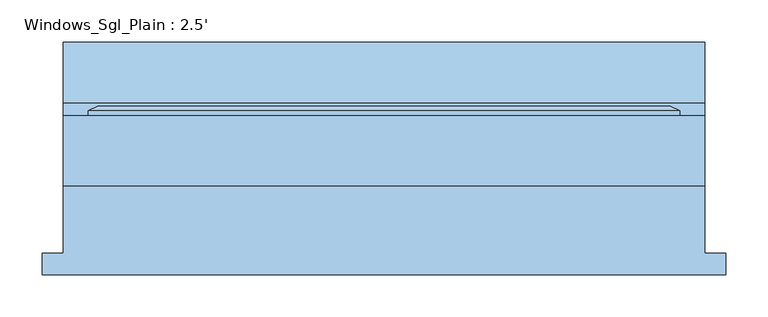
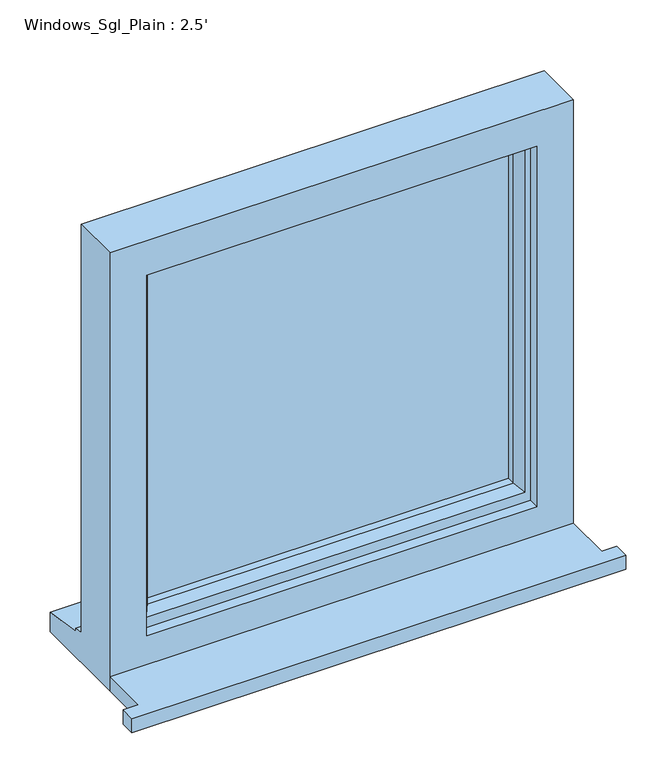
"""IFC4 building model written with IfcOpenShell, lengths in millimetres: window geometry, Windows_Sgl_Plain : 2.5'."""

from ifc_helpers import new_model, si_unit, frame, origin, place, context, project, spatial, polyline, outline, extrude, faceted_brep, source, transform, mapped, element, save


def windows_sgl_plain_2_5_21186da1(model_context):
    return source(origin(), model_context, "Body", "SolidModel", [
        extrude(outline(polyline([(-406.0, -123.2234322), (-406.0, -98.2234322), (-381.0, -98.2234322), (-381.0, -17.8634322), (381.0, -17.8634322), (381.0, -98.2234322), (406.0, -98.2234322), (406.0, -123.2234322), (-406.0, -123.2234322)])), frame((0.0, 0.0, 1348.0), z_axis=(0.0, 0.0, 1.0), x_axis=(1.0, 0.0, 0.0)), (0.0, 0.0, 1.0), 25.0),
        faceted_brep([(-381.0, -17.8634322, 1348.0), (381.0, -17.8634322, 1348.0), (381.0, -17.8634322, 2110.0), (-381.0, -17.8634322, 2110.0), (-321.0, -17.8634322, 2050.0), (321.0, -17.8634322, 2050.0), (321.0, -17.8634322, 1423.0), (-321.0, -17.8634322, 1423.0), (-381.0, 65.1365678, 2110.0), (-381.0, 65.1365678, 1399.0), (-381.0, 80.1365678, 1397.68767), (-381.0, 80.1365678, 1392.7449676), (-381.0, 152.6365678, 1381.8088847), (-381.0, 152.6365678, 1348.0), (381.0, 65.1365678, 2110.0), (381.0, 65.1365678, 1399.0), (-341.0, 65.1365678, 2070.0), (-341.0, 65.1365678, 1411.0), (341.0, 65.1365678, 1411.0), (341.0, 65.1365678, 2070.0), (-341.0, 0.1365678, 2070.0), (-341.0, 0.1365678, 1411.0), (341.0, 0.1365678, 2070.0), (341.0, 0.1365678, 1411.0), (-321.0, 0.1365678, 2050.0), (-321.0, 0.1365678, 1423.0), (321.0, 0.1365678, 1423.0), (321.0, 0.1365678, 2050.0), (381.0, 152.6365678, 1348.0), (381.0, 152.6365678, 1381.8088847), (381.0, 80.1365678, 1392.7449676), (381.0, 80.1365678, 1397.68767)], [[[0, 1, 2, 3], [4, 5, 6, 7]], [[0, 3, 8, 9, 10, 11, 12, 13]], [[9, 8, 14, 15], [16, 17, 18, 19]], [[17, 16, 20, 21]], [[20, 22, 23, 21], [24, 25, 26, 27]], [[24, 4, 7, 25]], [[3, 2, 14, 8]], [[16, 19, 22, 20]], [[5, 4, 24, 27]], [[15, 14, 2, 1, 28, 29, 30, 31]], [[19, 18, 23, 22]], [[5, 27, 26, 6]], [[28, 1, 0, 13]], [[29, 28, 13, 12]], [[30, 29, 12, 11]], [[31, 30, 11, 10]], [[15, 31, 10, 9]], [[21, 23, 18, 17]], [[7, 6, 26, 25]]]),
        extrude(outline(polyline([(311.0, 29.1365678), (-311.0, 29.1365678), (-311.0, 53.1365678), (311.0, 53.1365678), (311.0, 29.1365678)])), frame((0.0, 0.0, 1441.0), z_axis=(0.0, 0.0, 1.0), x_axis=(1.0, 0.0, 0.0)), (0.0, 0.0, 1.0), 599.0),
        faceted_brep([(-351.0, 65.1365678, 2080.0), (-351.0, 70.9100705, 2080.0), (-351.0, 70.9100705, 1401.0), (-351.0, 65.1365678, 1401.0), (-341.0, 0.1365678, 2070.0), (-341.0, 65.1365678, 2070.0), (-341.0, 65.1365678, 1411.0), (-341.0, 0.1365678, 1411.0), (-301.0, 14.6294677, 2030.0), (-311.1480377, 0.1365678, 2040.1480377), (-311.1480377, 0.1365678, 1440.8519623), (-301.0, 14.6294677, 1451.0), (-301.0, 29.1365678, 2030.0), (-301.0, 29.1365678, 1451.0), (-311.0, 53.1365678, 2040.0), (-311.0, 29.1365678, 2040.0), (-311.0, 29.1365678, 1441.0), (-311.0, 53.1365678, 1441.0), (-301.0, 70.9100705, 2030.0), (-301.0, 53.1365678, 2030.0), (-301.0, 53.1365678, 1451.0), (-301.0, 70.9100705, 1451.0), (-318.4457548, 76.6835732, 2047.4457548), (-318.4457548, 76.6835732, 1433.5542452), (-340.2153903, 76.6835732, 2069.2153903), (-340.2153903, 76.6835732, 1411.7846097), (351.0, 70.9100705, 1401.0), (351.0, 65.1365678, 1401.0), (341.0, 65.1365678, 1411.0), (341.0, 0.1365678, 1411.0), (311.1480377, 0.1365678, 1440.8519623), (301.0, 14.6294677, 1451.0), (301.0, 29.1365678, 1451.0), (311.0, 29.1365678, 1441.0), (311.0, 53.1365678, 1441.0), (301.0, 53.1365678, 1451.0), (301.0, 70.9100705, 1451.0), (318.4457548, 76.6835732, 1433.5542452), (340.2153903, 76.6835732, 1411.7846097), (351.0, 70.9100705, 2080.0), (351.0, 65.1365678, 2080.0), (341.0, 65.1365678, 2070.0), (341.0, 0.1365678, 2070.0), (311.1480377, 0.1365678, 2040.1480377), (301.0, 14.6294677, 2030.0), (301.0, 29.1365678, 2030.0), (311.0, 29.1365678, 2040.0), (311.0, 53.1365678, 2040.0), (301.0, 53.1365678, 2030.0), (301.0, 70.9100705, 2030.0), (318.4457548, 76.6835732, 2047.4457548), (340.2153903, 76.6835732, 2069.2153903)], [[[0, 1, 2, 3]], [[4, 5, 6, 7]], [[8, 9, 10, 11]], [[12, 8, 11, 13]], [[14, 15, 16, 17]], [[18, 19, 20, 21]], [[22, 18, 21, 23]], [[1, 24, 25, 2]], [[3, 2, 26, 27]], [[7, 6, 28, 29]], [[11, 10, 30, 31]], [[13, 11, 31, 32]], [[17, 16, 33, 34]], [[21, 20, 35, 36]], [[23, 21, 36, 37]], [[2, 25, 38, 26]], [[27, 26, 39, 40]], [[29, 28, 41, 42]], [[31, 30, 43, 44]], [[32, 31, 44, 45]], [[34, 33, 46, 47]], [[36, 35, 48, 49]], [[37, 36, 49, 50]], [[26, 38, 51, 39]], [[40, 39, 1, 0]], [[3, 27, 40, 0], [5, 41, 28, 6]], [[42, 41, 5, 4]], [[7, 29, 42, 4], [9, 43, 30, 10]], [[44, 43, 9, 8]], [[45, 44, 8, 12]], [[15, 46, 33, 16], [13, 32, 45, 12]], [[47, 46, 15, 14]], [[17, 34, 47, 14], [19, 48, 35, 20]], [[49, 48, 19, 18]], [[50, 49, 18, 22]], [[24, 51, 38, 25], [23, 37, 50, 22]], [[39, 51, 24, 1]]]),
    ])


if __name__ == "__main__":
    model = new_model("IFC4")
    model_context = context("Model", 3, world=origin())
    ifc_project = project(units=[si_unit("LENGTHUNIT", "METRE", prefix="MILLI")], contexts=[model_context])
    site = spatial("IfcSite", under=ifc_project)
    building = spatial("IfcBuilding", under=site)
    placement = place(None, origin())
    windows_sgl_plain_2_5_shape = windows_sgl_plain_2_5_21186da1(model_context)
    element("IfcWindow", 1, ObjectType="Windows_Sgl_Plain : 2.5'", at=placement, inside=building, context=model_context, shape_type="MappedRepresentation", body=[
        mapped(windows_sgl_plain_2_5_shape, transform((0.0, 0.0, 0.0), x_axis=(1.0, 0.0, 0.0), y_axis=(0.0, 1.0, 0.0), z_axis=(0.0, 0.0, 1.0))),
    ])
    save(model, "model.ifc")

# Revit data of these elements
# Type "Windows_Sgl_Plain : 2.5'"
#   Type Mark = "61"
#   Operation = "SinglePanel"
#   Construction Type Id = "SGL"
#   Manufacturer = "Revit"
#   Keynote = "L10"
#   Analytic Construction = "Large single-glazed windows"
#   Wrap Layers (Ext) from Ext = 0.336286 ft
#   Wrap Layers (Int) from Ext = 0.582349 ft
#   Window Board Projection = 0.082021 ft
#   Window Board Extension = 0.082021 ft
#   Visual Light Transmittance = 0.9
#   Solar Heat Gain Coefficient = 0.86
#   Rough Width = 2.5 ft
#   Rough Height = 2.5 ft
#   Height = 2.5 ft
#   Width = 2.5 ft
#   Heat Transfer Coefficient (U) = 5.5617 W/(m²·K)
#   Glazing Thickness = 0.07874 ft
#   FrameOffset - External = 0.164042 ft
#   Frame Depth = 0.213255 ft
#   Default Head Height = 6.922572 ft
#   Cill Depth = 0.287073 ft
#   Cavity Closer Width = 0.164042 ft
#   Cavity Closer Offset from Ext = 0.336286 ft
#   Cavity Closer Depth = 0.278871 ft
#   Vis - Cavity Closers = yes
#   Define Thermal Properties by = 1
#   Material Trim = Window Frame
#   Material Glass = Glass
#   Material Frame = Window Frame
#   Wall Closure = (empty or 0)
# Element 1 (IfcWindow, "Windows_Sgl_Plain : 2.5'")
#   Materials on its faces: "Window Frame", "Glass"
# Materials
#   "Window Frame": colour RGB 249 249 249, transparency 0, Keynote = "L10", Cost = 0
#   "Glass": class "Glass", colour RGB 0 128 192, transparency 0.9, Description = "Soda Lime Glass", Cost = 0
